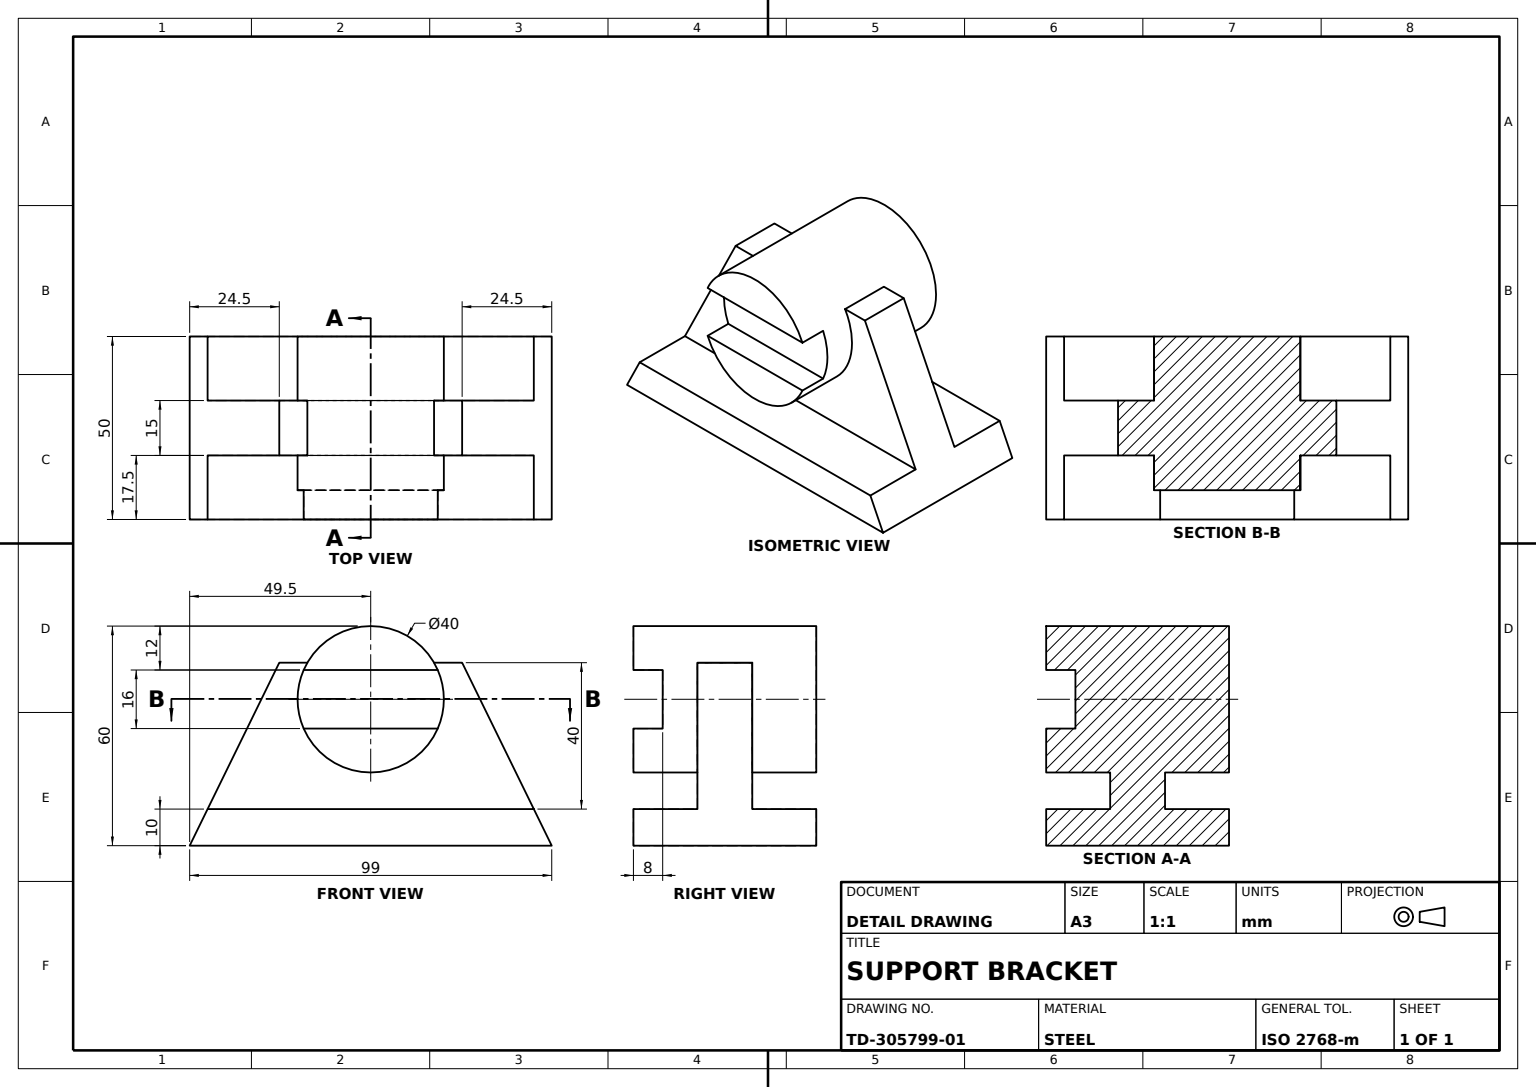
SolidWorks part; units mm, degrees
material "Plain Carbon Steel"
ref_plane "Front Plane" through (0, 0, 0) normal (0, 0, 1) x (1, 0, 0)
ref_plane "Top Plane" through (0, 0, 0) normal (0, 1, 0) x (1, 0, 0)
ref_plane "Right Plane" through (0, 0, 0) normal (1, 0, 0) x (0, 0, -1)
sketch "Base Plate Sketch" plane through (0, 0, 0) normal (0, 1, 0) x (1, 0, 0)
  line L1 (-49.5, 25) -> (49.5, 25)
  line L2 (-49.5, 25) -> (-49.5, -25)
  line L3 (-49.5, -25) -> (49.5, -25)
  line L4 (49.5, 25) -> (49.5, -25)
  line L5 (-49.5, 25) -> (49.5, -25) construction
  line L6 (-49.5, -25) -> (49.5, 25) construction
  point P0 (0, 0)
  dimension "D1" = 99
  dimension "D2" = 50
extrude "Base Plate" add sketch "Base Plate Sketch" along normal blind 10
sketch "Support Block Sketch" plane through (0, 10, 0) normal (0, 1, 0) x (1, 0, 0)
  line L0 (-49.5, 25) -> (-49.5, -25) construction
  line L1 (-49.5, 7.5) -> (49.5, 7.5)
  line L2 (-49.5, 7.5) -> (-49.5, -7.5)
  line L3 (-49.5, -7.5) -> (49.5, -7.5)
  line L4 (49.5, 7.5) -> (49.5, -7.5)
  line L5 (49.5, -25) -> (49.5, 25) construction
  line L6 (49.5, 25) -> (-49.5, 25) construction
  dimension "D1" = 15
  dimension "D2" = 17.5
extrude "Support Block" add sketch "Support Block Sketch" along normal blind 40
sketch "Support Taper Sketch" plane through (0, 0, 0) normal (0, 0, 1) x (1, 0, 0)
  line L1 (-49.5, 50) -> (49.5, 50) construction
  line L2 (49.5, 50) -> (49.5, 10) construction
  line L3 (-49.5, 50) -> (-49.5, 10) construction
  line L4 (-25, 50) -> (-49.5, 0)
  line L5 (-49.5, 0) -> (-49.5, 50)
  line L6 (-49.5, 50) -> (-25, 50)
  line L7 (25, 50) -> (49.5, 0)
  line L8 (49.5, 0) -> (49.5, 50)
  line L9 (49.5, 50) -> (25, 50)
  dimension "D1" = 50
  dimension "D2" = 24.5
  dimension "D3" = 24.5
extrude "Support Taper Cut" cut sketch "Support Taper Sketch" against normal mid plane 80
sketch "Cylinder Boss Sketch" plane through (0, 0, 0) normal (0, 0, 1) x (1, 0, 0)
  line L0 (-25, 50) -> (25, 50) construction
  circle A0 centre (0, 40) radius 20
  dimension "D2" = 40
  dimension "D1" = 10
extrude "Cylinder Boss Ø40" add sketch "Cylinder Boss Sketch" along normal mid plane 50
sketch "End Slot Sketch" plane through (0, 0, 25) normal (0, 0, 1) x (1, 0, 0)
  line L1 (-23.6639, 48) -> (23.6639, 48)
  line L2 (-23.6639, 48) -> (-23.6639, 32)
  line L3 (-23.6639, 32) -> (23.6639, 32)
  line L4 (23.6639, 48) -> (23.6639, 32)
  line L5 (-23.6639, 48) -> (23.6639, 32) construction
  line L6 (-23.6639, 32) -> (23.6639, 48) construction
  circle A0 centre (0, 40) radius 20 construction
  point P0 (0, 40)
  dimension "D1" = 16
  dimension "D2" = 23.6639
extrude "End Slot 16x8" cut sketch "End Slot Sketch" against normal blind 8
